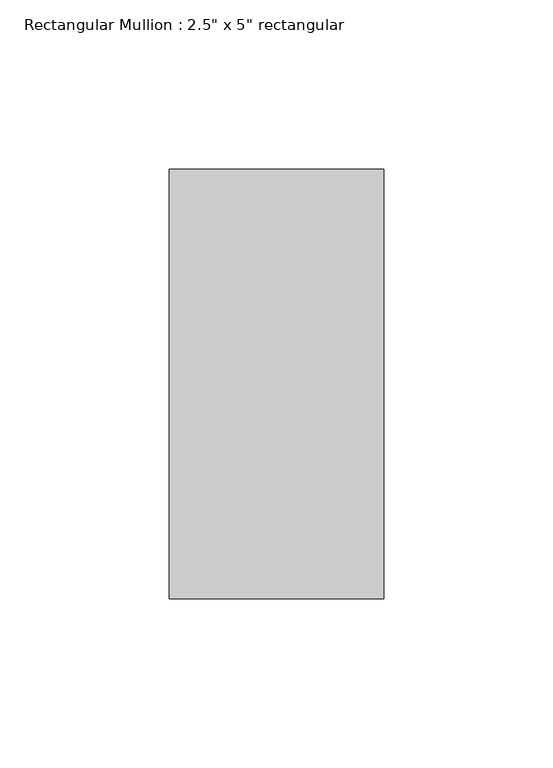
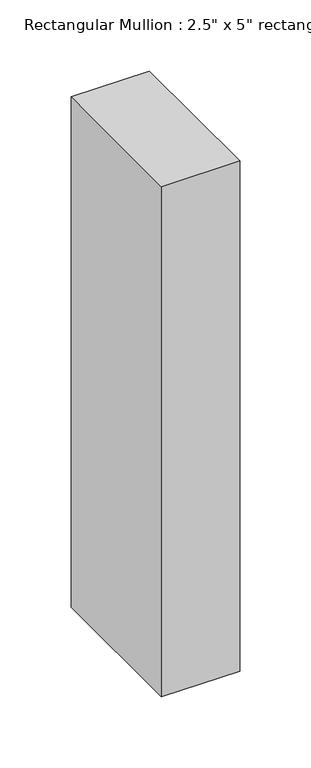
"""IFC4 building model written with IfcOpenShell, lengths in millimetres: member geometry."""

from ifc_helpers import new_model, si_unit, frame, origin, place, context, project, spatial, polyline, outline, extrude, source, transform, mapped, element, save


def member_6fb4a552(model_context):
    return source(origin(), model_context, "Body", "SweptSolid", [
        extrude(outline(polyline([(0.0, 63.5), (0.0, -63.5), (-63.5, -63.5), (-63.5, 63.5), (0.0, 63.5)])), frame((0.0, 0.0, -438.15), z_axis=(0.0, 0.0, 1.0), x_axis=(1.0, 0.0, 0.0)), (0.0, 0.0, 1.0), 438.15),
    ])


if __name__ == "__main__":
    model = new_model("IFC4")
    model_context = context("Model", 3, world=origin())
    ifc_project = project(units=[si_unit("LENGTHUNIT", "METRE", prefix="MILLI")], contexts=[model_context])
    site = spatial("IfcSite", under=ifc_project)
    building = spatial("IfcBuilding", under=site)
    placement = place(None, origin())
    member_shape = member_6fb4a552(model_context)
    element("IfcMember", 1, ObjectType="Rectangular Mullion : 2.5\" x 5\" rectangular", at=placement, inside=building, context=model_context, shape_type="MappedRepresentation", body=[
        mapped(member_shape, transform((0.0, 0.0, 0.0), x_axis=(1.0, 0.0, 0.0), y_axis=(0.0, 1.0, 0.0), z_axis=(0.0, 0.0, 1.0))),
    ])
    save(model, "model.ifc")

# Revit data of these elements
# Type "Rectangular Mullion : 2.5\" x 5\" rectangular"
#   built-in parameter 1007304 = 0.416667 (stored number, unit not read)
#   built-in parameter 1007301 = 0.104167 (stored number, unit not read)
#   built-in parameter 1007300 = 0.104167 (stored number, unit not read)
# Element 1 (IfcMember, "Rectangular Mullion : 2.5\" x 5\" rectangular")
#   Materials on its faces: "Rectangle 1 sq"
# Materials
#   "Rectangle 1 sq": class "Generic", colour RGB 120 120 120, transparency 0, Cost = 0
